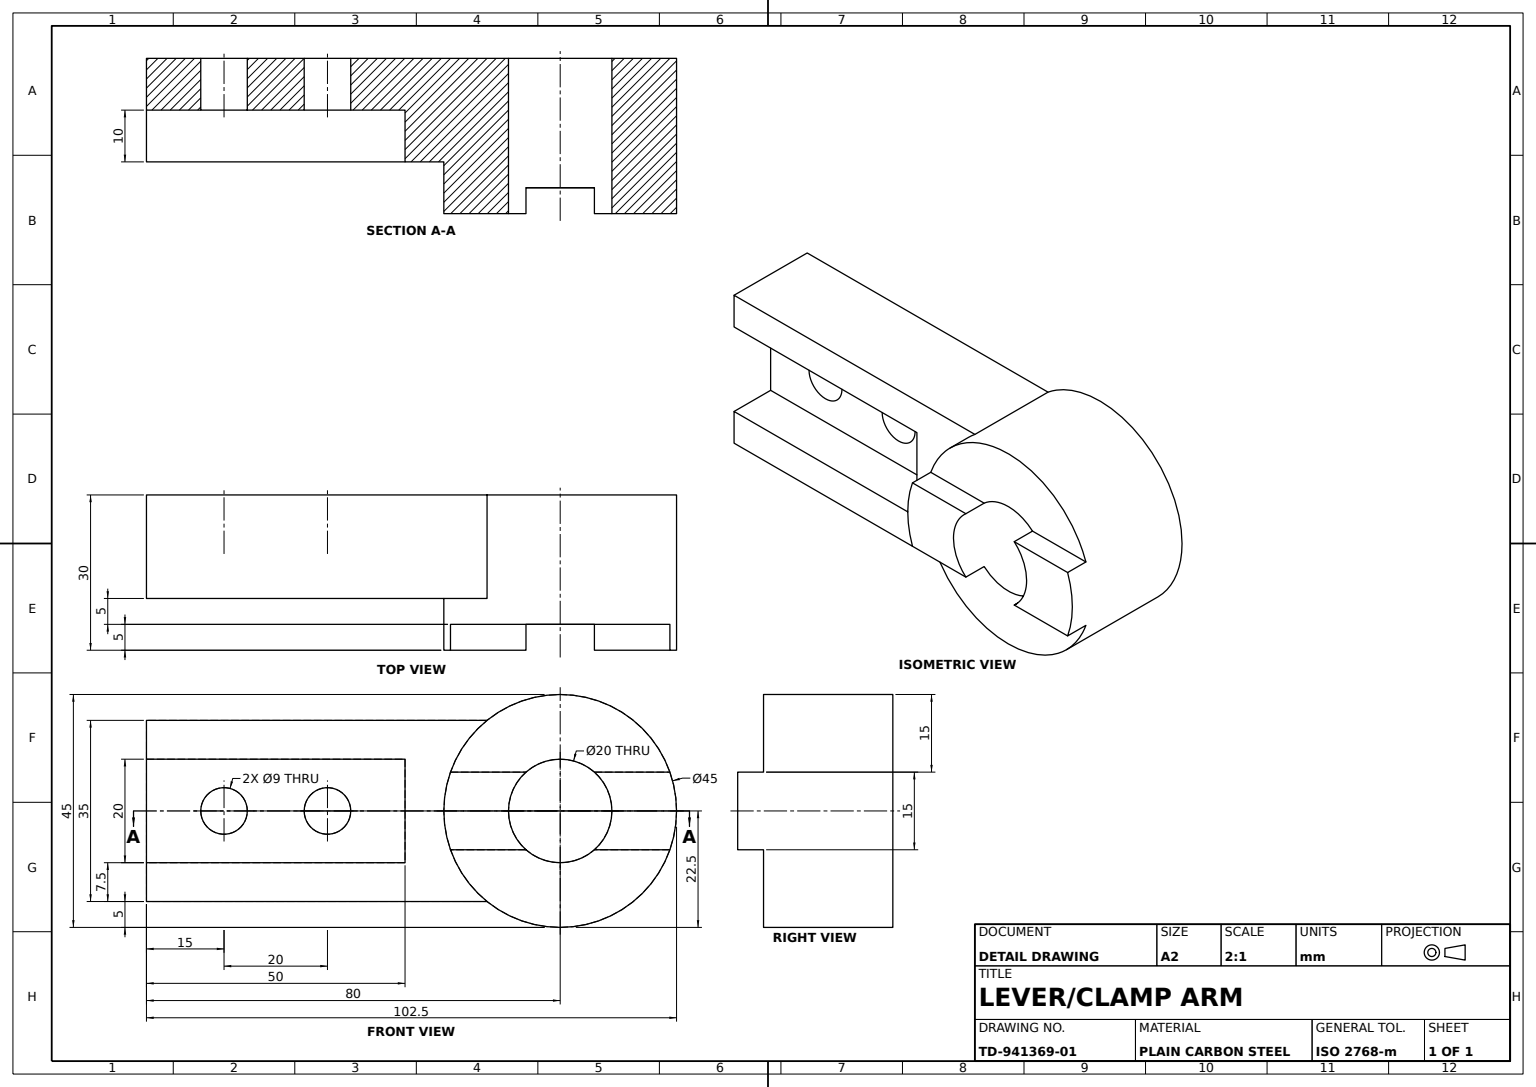
from build123d import *

# Parameters (mm, degrees)
HUB_PROFILE_SKETCH_R       = 22.5
HUB_PROFILE_SKETCH_R_2     = 10
HUB_BOSS_45_DEPTH          = 30
HUB_START                  = -5
HUB_FACE_SLOT_15_DEPTH     = 5
HUB_SLOT_STEP_15_DEPTH     = 5
CRANK_ARM_PROFILE_SKETCH_W = 20
CRANK_ARM_PROFILE_SKETCH_H = 35
CRANK_ARM_DEPTH            = 80
BORE_START                 = -80
BORE_SKETCH_R              = 10
BORE_20_DEPTH              = 80
ARM_WINDOW_SKETCH_W        = 10
ARM_WINDOW_SKETCH_H        = 20
ARM_WINDOW_10X20_DEPTH     = 50
ARM_SIDE_CUT_SKETCH_R      = 4.5
ARM_SIDE_CUT_DEPTH         = 86.476604986


with BuildPart() as part:
    # Hub Profile Sketch → Hub Boss Ø45 (new body)
    with BuildSketch(Plane(origin=(0, 0, 0), x_dir=(0, 0, -1), z_dir=(1, 0, 0))):
        Circle(HUB_PROFILE_SKETCH_R)
        Circle(HUB_PROFILE_SKETCH_R_2, mode=Mode.SUBTRACT)
    extrude(amount=HUB_BOSS_45_DEPTH)

    # Hub Face Slot Sketch → Hub Face Slot 15 (cut)
    with BuildSketch(Plane(origin=(30, 0, 0), x_dir=(0, 0, -1), z_dir=(1, 0, 0)).offset(HUB_START)):
        with BuildLine():
            Line((-21.213203436, 7.5), (21.213203436, 7.5))
            ThreePointArc((21.213203436, 7.5), (0, 22.5), (-21.213203436, 7.5))
        make_face()
    extrude(amount=HUB_FACE_SLOT_15_DEPTH, mode=Mode.SUBTRACT)

    # Hub Slot Step Sketch → Hub Slot Step 15 (cut)
    with BuildSketch(Plane(origin=(30, 0, 0), x_dir=(0, 0, -1), z_dir=(1, 0, 0)).offset(HUB_START)):
        with BuildLine():
            Line((-21.213203436, -7.5), (21.213203436, -7.5))
            ThreePointArc((21.213203436, -7.5), (0, -22.5), (-21.213203436, -7.5))
        make_face()
    extrude(amount=HUB_SLOT_STEP_15_DEPTH, mode=Mode.SUBTRACT)

    # Crank Arm Profile Sketch → Crank Arm (add)
    with BuildSketch(Plane.XY):
        with Locations((10, 0)):
            Rectangle(CRANK_ARM_PROFILE_SKETCH_W, CRANK_ARM_PROFILE_SKETCH_H)
    extrude(amount=CRANK_ARM_DEPTH)

    # Bore Sketch → Bore Ø20 (cut)
    with BuildSketch(Plane(origin=(20, 0, 0), x_dir=(0, 0, -1), z_dir=(1, 0, 0)).offset(BORE_START)):
        with Locations(Location((0, 0, 0), (0, 0, 131.409622109))):
            Circle(BORE_SKETCH_R)
    extrude(amount=BORE_20_DEPTH, mode=Mode.SUBTRACT)

    # Arm Window Sketch → Arm Window 10x20 (cut)
    with BuildSketch(Plane.XY.offset(80)):
        with Locations((15, 0)):
            Rectangle(ARM_WINDOW_SKETCH_W, ARM_WINDOW_SKETCH_H)
    extrude(amount=-ARM_WINDOW_10X20_DEPTH, mode=Mode.SUBTRACT)

    # Arm Side Cut Sketch → Arm Side Cut (cut, through all)
    with BuildSketch(Plane(origin=(10, 0, 0), x_dir=(0, 0, -1), z_dir=(1, 0, 0))):
        with Locations((-65, 0)):
            Circle(ARM_SIDE_CUT_SKETCH_R)
        with Locations((-45, 0)):
            Circle(ARM_SIDE_CUT_SKETCH_R)
    extrude(amount=-ARM_SIDE_CUT_DEPTH, mode=Mode.SUBTRACT)


solid = part.part
